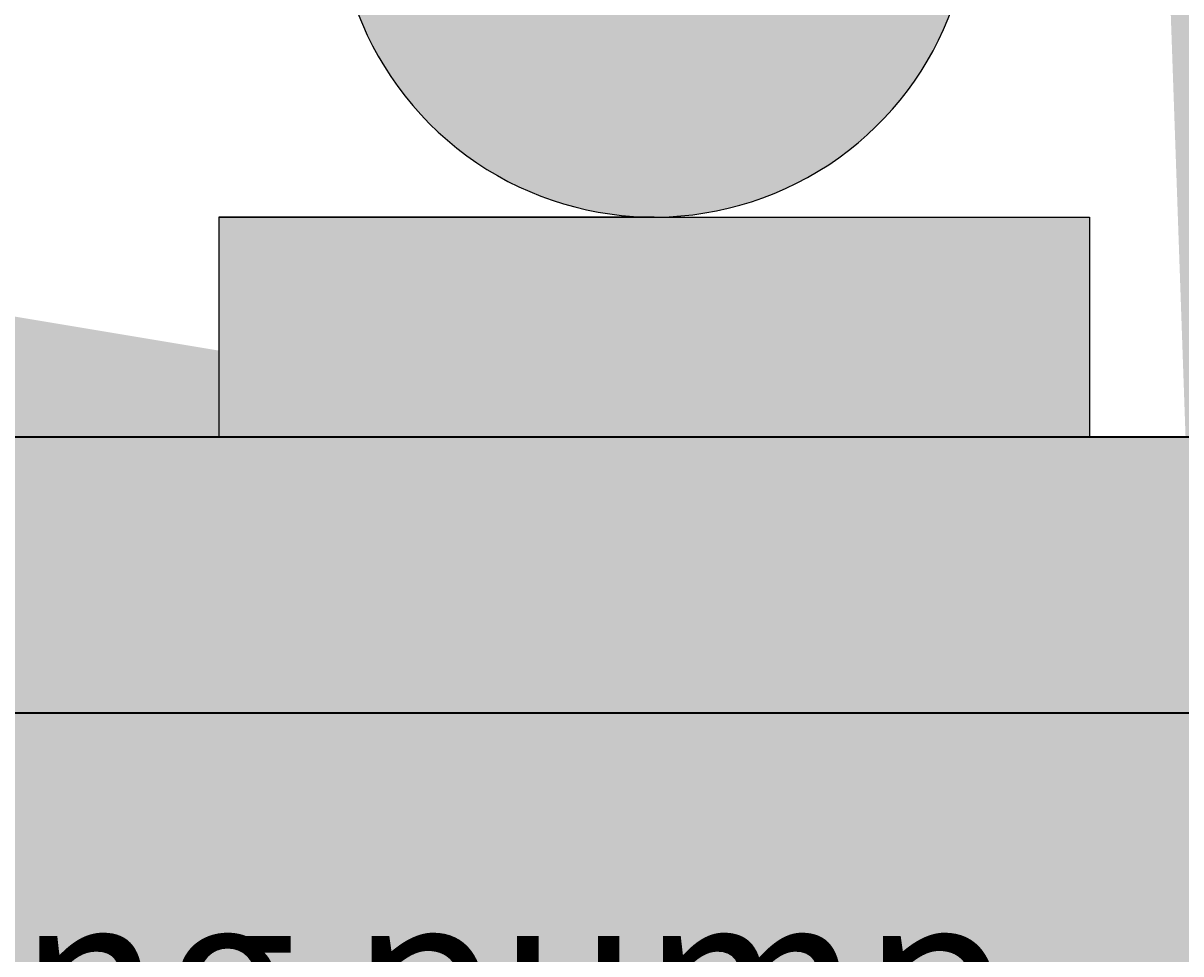
# Model space of a CAD drawing. Units: millimetres. Extents: x -22994 to 29398, y -19990 to 20176.
# Tile 10 of 135: x 32 to 58, y 5 to 26. Entities that reach past the tile are written whole.
import ezdxf
from ezdxf import colors
from ezdxf.entities.mleader import LeaderData, LeaderLine
from ezdxf.math import Vec2, Vec3

# ---------------------------------------------------------------- set-up
doc = ezdxf.new("R2010")
doc.units = ezdxf.units.MM
doc.header["$MEASUREMENT"] = 0
for name, color, linetype, lineweight in [('M-ANNO-TEXT', 7, 'Continuous', 25), ('M-DIMS', 2, 'Continuous', 18), ('M-EQPM', 7, 'Continuous', 25), ('M-EQPM-PATT', 7, 'Continuous', 18), ('S-FNDN', 7, 'Continuous', 35)]:
    doc.layers.add(name, color=color, linetype=linetype, lineweight=lineweight)
doc.styles.get("Standard").update_dxf_attribs({"font": 'arial.ttf'})
doc.dimstyles.get("Standard").update_dxf_attribs({"dimtxt": 0.18, "dimasz": 10000, "dimexe": 0.18, "dimexo": 0.0625, "dimgap": 0.09, "dimtad": 0, "dimtih": 1, "dimtoh": 1, "dimdec": 0, "dimzin": 0, "dimdsep": 46, "dimtxsty": 'Standard', "dimcen": 0.09, "dimadec": 0, "dimazin": 0, "dimtfac": 1, "dimtdec": 0, "dimtofl": 0, "dimtmove": 0, "dimatfit": 3, "dimfxl": 1, "dimtolj": 1, "dimtzin": 0, "dimlwd": 30, "dimarcsym": 0})

# ---------------------------------------------------------------- blocks, each defined once
blk = doc.blocks.new('*D2')
at = {"layer": 'Defpoints', "color": 0, "transparency": 16777216}
for p in [(6.677, 10.271), (290.852, 10.271), (290.852, -5.079)]:
    blk.add_point(p, dxfattribs=at)
at = {"layer": 'M-DIMS', "color": 0, "lineweight": -2, "transparency": 16777216}
for p, q in [((6.677, 10.209), (6.677, -5.259)), ((290.852, 10.209), (290.852, -5.259))]:
    blk.add_line(p, q, dxfattribs=at)
at = {"layer": 'M-DIMS', "color": 0, "lineweight": 30, "transparency": 16777216}
for p, q in [((-9993.323, -5.079), (-19993.323, -5.079)), ((10290.852, -5.079), (20290.852, -5.079))]:
    blk.add_line(p, q, dxfattribs=at)
at = {"layer": 'M-DIMS', "color": 0, "transparency": 16777216}
for points in [[(-9993.323, 1661.588), (-9993.323, -1671.745), (6.677, -5.079)], [(10290.852, 1661.588), (10290.852, -1671.745), (290.852, -5.079)]]:
    blk.add_solid(points, dxfattribs=at)
at = {"layer": 'M-DIMS', "color": 0, "transparency": 16777216, "insert": (148.765, -5.079), "char_height": 0.18, "attachment_point": 5}
blk.add_mtext('\\A1;284.2', dxfattribs=at)
blk = doc.blocks.new('*D3')
at = {"layer": 'Defpoints', "color": 0, "transparency": 16777216}
for p in [(110.265, 204.165), (110.265, 176.366), (95.833, 127.967)]:
    blk.add_point(p, dxfattribs=at)
at = {"layer": 'M-DIMS', "color": 0, "lineweight": -2, "transparency": 16777216}
for p, q in [((95.833, 128.03), (95.833, 204.345)), ((110.265, 176.429), (110.265, 204.345))]:
    blk.add_line(p, q, dxfattribs=at)
at = {"layer": 'M-DIMS', "color": 0, "lineweight": 30, "transparency": 16777216}
for p, q in [((-9904.167, 204.165), (-19904.167, 204.165)), ((10110.265, 204.165), (20110.265, 204.165))]:
    blk.add_line(p, q, dxfattribs=at)
at = {"layer": 'M-DIMS', "color": 0, "transparency": 16777216}
for points in [[(-9904.167, 1870.832), (-9904.167, -1462.501), (95.833, 204.165)], [(10110.265, 1870.832), (10110.265, -1462.501), (110.265, 204.165)]]:
    blk.add_solid(points, dxfattribs=at)
at = {"layer": 'M-DIMS', "color": 0, "transparency": 16777216, "insert": (103.049, 204.165), "char_height": 0.18, "attachment_point": 5}
blk.add_mtext('\\A1;14.432', dxfattribs=at)
blk = doc.blocks.new('*D4')
at = {"layer": 'Defpoints', "color": 0, "transparency": 16777216}
for p in [(116.265, 204.165), (110.265, 176.366), (116.265, 176.366)]:
    blk.add_point(p, dxfattribs=at)
at = {"layer": 'M-DIMS', "color": 0, "lineweight": -2, "transparency": 16777216}
for p, q in [((110.265, 176.429), (110.265, 204.345)), ((116.265, 176.429), (116.265, 204.345))]:
    blk.add_line(p, q, dxfattribs=at)
at = {"layer": 'M-DIMS', "color": 0, "lineweight": 30, "transparency": 16777216}
for p, q in [((-9889.735, 204.165), (-19889.735, 204.165)), ((10116.265, 204.165), (20116.265, 204.165))]:
    blk.add_line(p, q, dxfattribs=at)
at = {"layer": 'M-DIMS', "color": 0, "transparency": 16777216}
for points in [[(-9889.735, 1870.832), (-9889.735, -1462.501), (110.265, 204.165)], [(10116.265, 1870.832), (10116.265, -1462.501), (116.265, 204.165)]]:
    blk.add_solid(points, dxfattribs=at)
at = {"layer": 'M-DIMS', "color": 0, "transparency": 16777216, "insert": (113.265, 204.165), "char_height": 0.18, "attachment_point": 5}
blk.add_mtext('\\A1;6', dxfattribs=at)
blk = doc.blocks.new('*D5')
at = {"layer": 'Defpoints', "color": 0, "transparency": 16777216}
for p in [(181.265, 204.165), (116.265, 176.366), (181.265, 176.366)]:
    blk.add_point(p, dxfattribs=at)
at = {"layer": 'M-DIMS', "color": 0, "lineweight": -2, "transparency": 16777216}
for p, q in [((116.265, 176.429), (116.265, 204.345)), ((181.265, 176.429), (181.265, 204.345))]:
    blk.add_line(p, q, dxfattribs=at)
at = {"layer": 'M-DIMS', "color": 0, "lineweight": 30, "transparency": 16777216}
for p, q in [((-9883.735, 204.165), (-19883.735, 204.165)), ((10181.265, 204.165), (20181.265, 204.165))]:
    blk.add_line(p, q, dxfattribs=at)
at = {"layer": 'M-DIMS', "color": 0, "transparency": 16777216}
for points in [[(-9883.735, 1870.832), (-9883.735, -1462.501), (116.265, 204.165)], [(10181.265, 1870.832), (10181.265, -1462.501), (181.265, 204.165)]]:
    blk.add_solid(points, dxfattribs=at)
at = {"layer": 'M-DIMS', "color": 0, "transparency": 16777216, "insert": (148.765, 204.165), "char_height": 0.18, "attachment_point": 5}
blk.add_mtext('\\A1;65', dxfattribs=at)
blk = doc.blocks.new('*D6')
at = {"layer": 'Defpoints', "color": 0, "transparency": 16777216}
for p in [(187.265, 204.165), (181.265, 176.366), (187.265, 176.366)]:
    blk.add_point(p, dxfattribs=at)
at = {"layer": 'M-DIMS', "color": 0, "lineweight": -2, "transparency": 16777216}
for p, q in [((181.265, 176.429), (181.265, 204.345)), ((187.265, 176.429), (187.265, 204.345))]:
    blk.add_line(p, q, dxfattribs=at)
at = {"layer": 'M-DIMS', "color": 0, "lineweight": 30, "transparency": 16777216}
for p, q in [((-9818.735, 204.165), (-19818.735, 204.165)), ((10187.265, 204.165), (20187.265, 204.165))]:
    blk.add_line(p, q, dxfattribs=at)
at = {"layer": 'M-DIMS', "color": 0, "transparency": 16777216}
for points in [[(-9818.735, 1870.832), (-9818.735, -1462.501), (181.265, 204.165)], [(10187.265, 1870.832), (10187.265, -1462.501), (187.265, 204.165)]]:
    blk.add_solid(points, dxfattribs=at)
at = {"layer": 'M-DIMS', "color": 0, "transparency": 16777216, "insert": (184.265, 204.165), "char_height": 0.18, "attachment_point": 5}
blk.add_mtext('\\A1;6', dxfattribs=at)
blk = doc.blocks.new('*D7')
at = {"layer": 'Defpoints', "color": 0, "transparency": 16777216}
for p in [(201.697, 204.165), (187.265, 176.366), (201.697, 127.967)]:
    blk.add_point(p, dxfattribs=at)
at = {"layer": 'M-DIMS', "color": 0, "lineweight": -2, "transparency": 16777216}
for p, q in [((187.265, 176.429), (187.265, 204.345)), ((201.697, 128.03), (201.697, 204.345))]:
    blk.add_line(p, q, dxfattribs=at)
at = {"layer": 'M-DIMS', "color": 0, "lineweight": 30, "transparency": 16777216}
for p, q in [((-9812.735, 204.165), (-19812.735, 204.165)), ((10201.697, 204.165), (20201.697, 204.165))]:
    blk.add_line(p, q, dxfattribs=at)
at = {"layer": 'M-DIMS', "color": 0, "transparency": 16777216}
for points in [[(-9812.735, 1870.832), (-9812.735, -1462.501), (187.265, 204.165)], [(10201.697, 1870.832), (10201.697, -1462.501), (201.697, 204.165)]]:
    blk.add_solid(points, dxfattribs=at)
at = {"layer": 'M-DIMS', "color": 0, "transparency": 16777216, "insert": (194.481, 204.165), "char_height": 0.18, "attachment_point": 5}
blk.add_mtext('\\A1;14.432', dxfattribs=at)
blk = doc.blocks.new('*D8')
at = {"layer": 'Defpoints', "color": 0, "transparency": 16777216}
for p in [(227.648, 204.165), (227.648, 146.73), (201.697, 127.967)]:
    blk.add_point(p, dxfattribs=at)
at = {"layer": 'M-DIMS', "color": 0, "lineweight": -2, "transparency": 16777216}
for p, q in [((201.697, 128.03), (201.697, 204.345)), ((227.648, 146.792), (227.648, 204.345))]:
    blk.add_line(p, q, dxfattribs=at)
at = {"layer": 'M-DIMS', "color": 0, "lineweight": 30, "transparency": 16777216}
for p, q in [((-9798.303, 204.165), (-19798.303, 204.165)), ((10227.648, 204.165), (20227.648, 204.165))]:
    blk.add_line(p, q, dxfattribs=at)
at = {"layer": 'M-DIMS', "color": 0, "transparency": 16777216}
for points in [[(-9798.303, 1870.832), (-9798.303, -1462.501), (201.697, 204.165)], [(10227.648, 1870.832), (10227.648, -1462.501), (227.648, 204.165)]]:
    blk.add_solid(points, dxfattribs=at)
at = {"layer": 'M-DIMS', "color": 0, "transparency": 16777216, "insert": (214.673, 204.165), "char_height": 0.18, "attachment_point": 5}
blk.add_mtext('\\A1;25.95', dxfattribs=at)
blk = doc.blocks.new('*D9')
at = {"layer": 'Defpoints', "color": 0, "transparency": 16777216}
for p in [(187.265, 176.366), (306.202, 176.366), (290.852, 10.271)]:
    blk.add_point(p, dxfattribs=at)
at = {"layer": 'M-DIMS', "color": 0, "lineweight": 30, "transparency": 16777216}
for p, q in [((306.202, 10176.366), (306.202, 20176.366)), ((306.202, -9989.729), (306.202, -19989.729))]:
    blk.add_line(p, q, dxfattribs=at)
at = {"layer": 'M-DIMS', "color": 0, "lineweight": -2, "transparency": 16777216}
for p, q in [((187.327, 176.366), (306.382, 176.366)), ((290.915, 10.271), (306.382, 10.271))]:
    blk.add_line(p, q, dxfattribs=at)
at = {"layer": 'M-DIMS', "color": 0, "transparency": 16777216}
for points in [[(-1360.465, 10176.366), (1972.869, 10176.366), (306.202, 176.366)], [(-1360.465, -9989.729), (1972.869, -9989.729), (306.202, 10.271)]]:
    blk.add_solid(points, dxfattribs=at)
at = {"layer": 'M-DIMS', "color": 0, "transparency": 16777216, "insert": (306.202, 93.319), "char_height": 0.18, "attachment_point": 5}
blk.add_mtext('\\A1;166.1', dxfattribs=at)
blk = doc.blocks.new('*D10')
at = {"layer": 'Defpoints', "color": 0, "transparency": 16777216}
for p in [(125.65, 136.071), (133.346, 136.071), (133.346, -5.079)]:
    blk.add_point(p, dxfattribs=at)
at = {"layer": 'M-DIMS', "color": 0, "lineweight": -2, "transparency": 16777216}
for p, q in [((125.65, 136.009), (125.65, -5.259)), ((133.346, 136.009), (133.346, -5.259))]:
    blk.add_line(p, q, dxfattribs=at)
at = {"layer": 'M-DIMS', "color": 0, "lineweight": 30, "transparency": 16777216}
for p, q in [((-9874.35, -5.079), (-19874.35, -5.079)), ((10133.346, -5.079), (20133.346, -5.079))]:
    blk.add_line(p, q, dxfattribs=at)
at = {"layer": 'M-DIMS', "color": 0, "transparency": 16777216}
for points in [[(-9874.35, 1661.588), (-9874.35, -1671.745), (125.65, -5.079)], [(10133.346, 1661.588), (10133.346, -1671.745), (133.346, -5.079)]]:
    blk.add_solid(points, dxfattribs=at)
at = {"layer": 'M-DIMS', "color": 0, "transparency": 16777216, "insert": (129.498, -5.079), "char_height": 0.18, "attachment_point": 5}
blk.add_mtext('\\A1;7.696', dxfattribs=at)
blk = doc.blocks.new('*D11')
at = {"layer": 'Defpoints', "color": 0, "transparency": 16777216}
for p in [(133.346, 136.071), (135.65, 136.071), (135.65, -5.079)]:
    blk.add_point(p, dxfattribs=at)
at = {"layer": 'M-DIMS', "color": 0, "lineweight": -2, "transparency": 16777216}
for p, q in [((133.346, 136.009), (133.346, -5.259)), ((135.65, 136.009), (135.65, -5.259))]:
    blk.add_line(p, q, dxfattribs=at)
at = {"layer": 'M-DIMS', "color": 0, "lineweight": 30, "transparency": 16777216}
for p, q in [((-9866.654, -5.079), (-19866.654, -5.079)), ((10135.65, -5.079), (20135.65, -5.079))]:
    blk.add_line(p, q, dxfattribs=at)
at = {"layer": 'M-DIMS', "color": 0, "transparency": 16777216}
for points in [[(-9866.654, 1661.588), (-9866.654, -1671.745), (133.346, -5.079)], [(10135.65, 1661.588), (10135.65, -1671.745), (135.65, -5.079)]]:
    blk.add_solid(points, dxfattribs=at)
at = {"layer": 'M-DIMS', "color": 0, "transparency": 16777216, "insert": (134.498, -5.079), "char_height": 0.18, "attachment_point": 5}
blk.add_mtext('\\A1;2.304', dxfattribs=at)
blk = doc.blocks.new('*D12')
at = {"layer": 'Defpoints', "color": 0, "transparency": 16777216}
for p in [(135.65, 136.071), (145.65, 136.071), (145.65, -5.079)]:
    blk.add_point(p, dxfattribs=at)
at = {"layer": 'M-DIMS', "color": 0, "lineweight": -2, "transparency": 16777216}
for p, q in [((135.65, 136.009), (135.65, -5.259)), ((145.65, 136.009), (145.65, -5.259))]:
    blk.add_line(p, q, dxfattribs=at)
at = {"layer": 'M-DIMS', "color": 0, "lineweight": 30, "transparency": 16777216}
for p, q in [((-9864.35, -5.079), (-19864.35, -5.079)), ((10145.65, -5.079), (20145.65, -5.079))]:
    blk.add_line(p, q, dxfattribs=at)
at = {"layer": 'M-DIMS', "color": 0, "transparency": 16777216}
for points in [[(-9864.35, 1661.588), (-9864.35, -1671.745), (135.65, -5.079)], [(10145.65, 1661.588), (10145.65, -1671.745), (145.65, -5.079)]]:
    blk.add_solid(points, dxfattribs=at)
at = {"layer": 'M-DIMS', "color": 0, "transparency": 16777216, "insert": (140.65, -5.079), "char_height": 0.18, "attachment_point": 5}
blk.add_mtext('\\A1;10', dxfattribs=at)
blk = doc.blocks.new('*D13')
at = {"layer": 'Defpoints', "color": 0, "transparency": 16777216}
for p in [(145.65, 136.071), (155.65, 136.071), (155.65, -5.079)]:
    blk.add_point(p, dxfattribs=at)
at = {"layer": 'M-DIMS', "color": 0, "lineweight": -2, "transparency": 16777216}
for p, q in [((145.65, 136.009), (145.65, -5.259)), ((155.65, 136.009), (155.65, -5.259))]:
    blk.add_line(p, q, dxfattribs=at)
at = {"layer": 'M-DIMS', "color": 0, "lineweight": 30, "transparency": 16777216}
for p, q in [((-9854.35, -5.079), (-19854.35, -5.079)), ((10155.65, -5.079), (20155.65, -5.079))]:
    blk.add_line(p, q, dxfattribs=at)
at = {"layer": 'M-DIMS', "color": 0, "transparency": 16777216}
for points in [[(-9854.35, 1661.588), (-9854.35, -1671.745), (145.65, -5.079)], [(10155.65, 1661.588), (10155.65, -1671.745), (155.65, -5.079)]]:
    blk.add_solid(points, dxfattribs=at)
at = {"layer": 'M-DIMS', "color": 0, "transparency": 16777216, "insert": (150.65, -5.079), "char_height": 0.18, "attachment_point": 5}
blk.add_mtext('\\A1;10', dxfattribs=at)
blk = doc.blocks.new('*D14')
at = {"layer": 'Defpoints', "color": 0, "transparency": 16777216}
for p in [(155.65, 136.071), (165.65, 136.071), (165.65, -5.079)]:
    blk.add_point(p, dxfattribs=at)
at = {"layer": 'M-DIMS', "color": 0, "lineweight": -2, "transparency": 16777216}
for p, q in [((155.65, 136.009), (155.65, -5.259)), ((165.65, 136.009), (165.65, -5.259))]:
    blk.add_line(p, q, dxfattribs=at)
at = {"layer": 'M-DIMS', "color": 0, "lineweight": 30, "transparency": 16777216}
for p, q in [((-9844.35, -5.079), (-19844.35, -5.079)), ((10165.65, -5.079), (20165.65, -5.079))]:
    blk.add_line(p, q, dxfattribs=at)
at = {"layer": 'M-DIMS', "color": 0, "transparency": 16777216}
for points in [[(-9844.35, 1661.588), (-9844.35, -1671.745), (155.65, -5.079)], [(10165.65, 1661.588), (10165.65, -1671.745), (165.65, -5.079)]]:
    blk.add_solid(points, dxfattribs=at)
at = {"layer": 'M-DIMS', "color": 0, "transparency": 16777216, "insert": (160.65, -5.079), "char_height": 0.18, "attachment_point": 5}
blk.add_mtext('\\A1;10', dxfattribs=at)
blk = doc.blocks.new('*D15')
at = {"layer": 'Defpoints', "color": 0, "transparency": 16777216}
for p in [(173.346, 154.788), (173.346, 136.071), (306.202, 136.071)]:
    blk.add_point(p, dxfattribs=at)
at = {"layer": 'M-DIMS', "color": 0, "lineweight": 30, "transparency": 16777216}
for p, q in [((306.202, 10154.788), (306.202, 20154.788)), ((306.202, -9863.929), (306.202, -19863.929))]:
    blk.add_line(p, q, dxfattribs=at)
at = {"layer": 'M-DIMS', "color": 0, "lineweight": -2, "transparency": 16777216}
for p, q in [((173.408, 154.788), (306.382, 154.788)), ((173.408, 136.071), (306.382, 136.071))]:
    blk.add_line(p, q, dxfattribs=at)
at = {"layer": 'M-DIMS', "color": 0, "transparency": 16777216}
for points in [[(-1360.465, 10154.788), (1972.869, 10154.788), (306.202, 154.788)], [(-1360.465, -9863.929), (1972.869, -9863.929), (306.202, 136.071)]]:
    blk.add_solid(points, dxfattribs=at)
at = {"layer": 'M-DIMS', "color": 0, "transparency": 16777216, "insert": (306.202, 145.43), "char_height": 0.18, "attachment_point": 5}
blk.add_mtext('\\A1;18.717', dxfattribs=at)
blk = doc.blocks.new('*D16')
at = {"layer": 'Defpoints', "color": 0, "transparency": 16777216}
for p in [(120.17, 204.165), (110.466, 48.035), (120.17, 48.035)]:
    blk.add_point(p, dxfattribs=at)
at = {"layer": 'M-DIMS', "color": 0, "lineweight": -2, "transparency": 16777216}
for p, q in [((110.466, 48.097), (110.466, 204.345)), ((120.17, 48.097), (120.17, 204.345))]:
    blk.add_line(p, q, dxfattribs=at)
at = {"layer": 'M-DIMS', "color": 0, "lineweight": 30, "transparency": 16777216}
for p, q in [((-9889.534, 204.165), (-19889.534, 204.165)), ((10120.17, 204.165), (20120.17, 204.165))]:
    blk.add_line(p, q, dxfattribs=at)
at = {"layer": 'M-DIMS', "color": 0, "transparency": 16777216}
for points in [[(-9889.534, 1870.832), (-9889.534, -1462.501), (110.466, 204.165)], [(10120.17, 1870.832), (10120.17, -1462.501), (120.17, 204.165)]]:
    blk.add_solid(points, dxfattribs=at)
at = {"layer": 'M-DIMS', "color": 0, "transparency": 16777216, "insert": (115.318, 204.165), "char_height": 0.18, "attachment_point": 5}
blk.add_mtext('\\A1;9.704', dxfattribs=at)
blk = doc.blocks.new('*D17')
at = {"layer": 'Defpoints', "color": 0, "transparency": 16777216}
for p in [(126.17, 204.165), (120.17, 48.035), (126.17, 48.035)]:
    blk.add_point(p, dxfattribs=at)
at = {"layer": 'M-DIMS', "color": 0, "lineweight": -2, "transparency": 16777216}
for p, q in [((120.17, 48.097), (120.17, 204.345)), ((126.17, 48.097), (126.17, 204.345))]:
    blk.add_line(p, q, dxfattribs=at)
at = {"layer": 'M-DIMS', "color": 0, "lineweight": 30, "transparency": 16777216}
for p, q in [((-9879.83, 204.165), (-19879.83, 204.165)), ((10126.17, 204.165), (20126.17, 204.165))]:
    blk.add_line(p, q, dxfattribs=at)
at = {"layer": 'M-DIMS', "color": 0, "transparency": 16777216}
for points in [[(-9879.83, 1870.832), (-9879.83, -1462.501), (120.17, 204.165)], [(10126.17, 1870.832), (10126.17, -1462.501), (126.17, 204.165)]]:
    blk.add_solid(points, dxfattribs=at)
at = {"layer": 'M-DIMS', "color": 0, "transparency": 16777216, "insert": (123.17, 204.165), "char_height": 0.18, "attachment_point": 5}
blk.add_mtext('\\A1;6', dxfattribs=at)
blk = doc.blocks.new('*D18')
at = {"layer": 'Defpoints', "color": 0, "transparency": 16777216}
for p in [(132.17, 204.165), (126.17, 48.035), (132.17, 48.035)]:
    blk.add_point(p, dxfattribs=at)
at = {"layer": 'M-DIMS', "color": 0, "lineweight": -2, "transparency": 16777216}
for p, q in [((126.17, 48.097), (126.17, 204.345)), ((132.17, 48.097), (132.17, 204.345))]:
    blk.add_line(p, q, dxfattribs=at)
at = {"layer": 'M-DIMS', "color": 0, "lineweight": 30, "transparency": 16777216}
for p, q in [((-9873.83, 204.165), (-19873.83, 204.165)), ((10132.17, 204.165), (20132.17, 204.165))]:
    blk.add_line(p, q, dxfattribs=at)
at = {"layer": 'M-DIMS', "color": 0, "transparency": 16777216}
for points in [[(-9873.83, 1870.832), (-9873.83, -1462.501), (126.17, 204.165)], [(10132.17, 1870.832), (10132.17, -1462.501), (132.17, 204.165)]]:
    blk.add_solid(points, dxfattribs=at)
at = {"layer": 'M-DIMS', "color": 0, "transparency": 16777216, "insert": (129.17, 204.165), "char_height": 0.18, "attachment_point": 5}
blk.add_mtext('\\A1;6', dxfattribs=at)
blk = doc.blocks.new('*D19')
at = {"layer": 'Defpoints', "color": 0, "transparency": 16777216}
for p in [(138.17, 204.165), (132.17, 48.035), (138.17, 48.035)]:
    blk.add_point(p, dxfattribs=at)
at = {"layer": 'M-DIMS', "color": 0, "lineweight": -2, "transparency": 16777216}
for p, q in [((132.17, 48.097), (132.17, 204.345)), ((138.17, 48.097), (138.17, 204.345))]:
    blk.add_line(p, q, dxfattribs=at)
at = {"layer": 'M-DIMS', "color": 0, "lineweight": 30, "transparency": 16777216}
for p, q in [((-9867.83, 204.165), (-19867.83, 204.165)), ((10138.17, 204.165), (20138.17, 204.165))]:
    blk.add_line(p, q, dxfattribs=at)
at = {"layer": 'M-DIMS', "color": 0, "transparency": 16777216}
for points in [[(-9867.83, 1870.832), (-9867.83, -1462.501), (132.17, 204.165)], [(10138.17, 1870.832), (10138.17, -1462.501), (138.17, 204.165)]]:
    blk.add_solid(points, dxfattribs=at)
at = {"layer": 'M-DIMS', "color": 0, "transparency": 16777216, "insert": (135.17, 204.165), "char_height": 0.18, "attachment_point": 5}
blk.add_mtext('\\A1;6', dxfattribs=at)
blk = doc.blocks.new('*D20')
at = {"layer": 'Defpoints', "color": 0, "transparency": 16777216}
for p in [(144.17, 204.165), (138.17, 48.035), (144.17, 48.035)]:
    blk.add_point(p, dxfattribs=at)
at = {"layer": 'M-DIMS', "color": 0, "lineweight": -2, "transparency": 16777216}
for p, q in [((138.17, 48.097), (138.17, 204.345)), ((144.17, 48.097), (144.17, 204.345))]:
    blk.add_line(p, q, dxfattribs=at)
at = {"layer": 'M-DIMS', "color": 0, "lineweight": 30, "transparency": 16777216}
for p, q in [((-9861.83, 204.165), (-19861.83, 204.165)), ((10144.17, 204.165), (20144.17, 204.165))]:
    blk.add_line(p, q, dxfattribs=at)
at = {"layer": 'M-DIMS', "color": 0, "transparency": 16777216}
for points in [[(-9861.83, 1870.832), (-9861.83, -1462.501), (138.17, 204.165)], [(10144.17, 1870.832), (10144.17, -1462.501), (144.17, 204.165)]]:
    blk.add_solid(points, dxfattribs=at)
at = {"layer": 'M-DIMS', "color": 0, "transparency": 16777216, "insert": (141.17, 204.165), "char_height": 0.18, "attachment_point": 5}
blk.add_mtext('\\A1;6', dxfattribs=at)
blk = doc.blocks.new('*D21')
at = {"layer": 'Defpoints', "color": 0, "transparency": 16777216}
for p in [(149.116, 204.165), (144.17, 48.035), (149.116, 48.035)]:
    blk.add_point(p, dxfattribs=at)
at = {"layer": 'M-DIMS', "color": 0, "lineweight": -2, "transparency": 16777216}
for p, q in [((144.17, 48.097), (144.17, 204.345)), ((149.116, 48.097), (149.116, 204.345))]:
    blk.add_line(p, q, dxfattribs=at)
at = {"layer": 'M-DIMS', "color": 0, "lineweight": 30, "transparency": 16777216}
for p, q in [((-9855.83, 204.165), (-19855.83, 204.165)), ((10149.116, 204.165), (20149.116, 204.165))]:
    blk.add_line(p, q, dxfattribs=at)
at = {"layer": 'M-DIMS', "color": 0, "transparency": 16777216}
for points in [[(-9855.83, 1870.832), (-9855.83, -1462.501), (144.17, 204.165)], [(10149.116, 1870.832), (10149.116, -1462.501), (149.116, 204.165)]]:
    blk.add_solid(points, dxfattribs=at)
at = {"layer": 'M-DIMS', "color": 0, "transparency": 16777216, "insert": (146.643, 204.165), "char_height": 0.18, "attachment_point": 5}
blk.add_mtext('\\A1;4.945', dxfattribs=at)
blk = doc.blocks.new('*D22')
at = {"layer": 'Defpoints', "color": 0, "transparency": 16777216}
for p in [(149.116, 30.99), (155.116, 30.99), (155.116, -5.079)]:
    blk.add_point(p, dxfattribs=at)
at = {"layer": 'M-DIMS', "color": 0, "lineweight": -2, "transparency": 16777216}
for p, q in [((149.116, 30.927), (149.116, -5.259)), ((155.116, 30.927), (155.116, -5.259))]:
    blk.add_line(p, q, dxfattribs=at)
at = {"layer": 'M-DIMS', "color": 0, "lineweight": 30, "transparency": 16777216}
for p, q in [((-9850.884, -5.079), (-19850.884, -5.079)), ((10155.116, -5.079), (20155.116, -5.079))]:
    blk.add_line(p, q, dxfattribs=at)
at = {"layer": 'M-DIMS', "color": 0, "transparency": 16777216}
for points in [[(-9850.884, 1661.588), (-9850.884, -1671.745), (149.116, -5.079)], [(10155.116, 1661.588), (10155.116, -1671.745), (155.116, -5.079)]]:
    blk.add_solid(points, dxfattribs=at)
at = {"layer": 'M-DIMS', "color": 0, "transparency": 16777216, "insert": (152.116, -5.079), "char_height": 0.18, "attachment_point": 5}
blk.add_mtext('\\A1;6', dxfattribs=at)
blk = doc.blocks.new('*D23')
at = {"layer": 'Defpoints', "color": 0, "transparency": 16777216}
for p in [(155.116, 30.99), (161.116, 30.99), (161.116, -5.079)]:
    blk.add_point(p, dxfattribs=at)
at = {"layer": 'M-DIMS', "color": 0, "lineweight": -2, "transparency": 16777216}
for p, q in [((155.116, 30.927), (155.116, -5.259)), ((161.116, 30.927), (161.116, -5.259))]:
    blk.add_line(p, q, dxfattribs=at)
at = {"layer": 'M-DIMS', "color": 0, "lineweight": 30, "transparency": 16777216}
for p, q in [((-9844.884, -5.079), (-19844.884, -5.079)), ((10161.116, -5.079), (20161.116, -5.079))]:
    blk.add_line(p, q, dxfattribs=at)
at = {"layer": 'M-DIMS', "color": 0, "transparency": 16777216}
for points in [[(-9844.884, 1661.588), (-9844.884, -1671.745), (155.116, -5.079)], [(10161.116, 1661.588), (10161.116, -1671.745), (161.116, -5.079)]]:
    blk.add_solid(points, dxfattribs=at)
at = {"layer": 'M-DIMS', "color": 0, "transparency": 16777216, "insert": (158.116, -5.079), "char_height": 0.18, "attachment_point": 5}
blk.add_mtext('\\A1;6', dxfattribs=at)
blk = doc.blocks.new('*D24')
at = {"layer": 'Defpoints', "color": 0, "transparency": 16777216}
for p in [(161.116, 30.99), (166.439, 30.99), (166.439, -5.079)]:
    blk.add_point(p, dxfattribs=at)
at = {"layer": 'M-DIMS', "color": 0, "lineweight": -2, "transparency": 16777216}
for p, q in [((161.116, 30.927), (161.116, -5.259)), ((166.439, 30.927), (166.439, -5.259))]:
    blk.add_line(p, q, dxfattribs=at)
at = {"layer": 'M-DIMS', "color": 0, "lineweight": 30, "transparency": 16777216}
for p, q in [((-9838.884, -5.079), (-19838.884, -5.079)), ((10166.439, -5.079), (20166.439, -5.079))]:
    blk.add_line(p, q, dxfattribs=at)
at = {"layer": 'M-DIMS', "color": 0, "transparency": 16777216}
for points in [[(-9838.884, 1661.588), (-9838.884, -1671.745), (161.116, -5.079)], [(10166.439, 1661.588), (10166.439, -1671.745), (166.439, -5.079)]]:
    blk.add_solid(points, dxfattribs=at)
at = {"layer": 'M-DIMS', "color": 0, "transparency": 16777216, "insert": (163.777, -5.079), "char_height": 0.18, "attachment_point": 5}
blk.add_mtext('\\A1;5.323', dxfattribs=at)
blk = doc.blocks.new('*D25')
at = {"layer": 'Defpoints', "color": 0, "transparency": 16777216}
for p in [(166.439, 30.99), (172.439, 30.99), (172.439, -5.079)]:
    blk.add_point(p, dxfattribs=at)
at = {"layer": 'M-DIMS', "color": 0, "lineweight": -2, "transparency": 16777216}
for p, q in [((166.439, 30.927), (166.439, -5.259)), ((172.439, 30.927), (172.439, -5.259))]:
    blk.add_line(p, q, dxfattribs=at)
at = {"layer": 'M-DIMS', "color": 0, "lineweight": 30, "transparency": 16777216}
for p, q in [((-9833.561, -5.079), (-19833.561, -5.079)), ((10172.439, -5.079), (20172.439, -5.079))]:
    blk.add_line(p, q, dxfattribs=at)
at = {"layer": 'M-DIMS', "color": 0, "transparency": 16777216}
for points in [[(-9833.561, 1661.588), (-9833.561, -1671.745), (166.439, -5.079)], [(10172.439, 1661.588), (10172.439, -1671.745), (172.439, -5.079)]]:
    blk.add_solid(points, dxfattribs=at)
at = {"layer": 'M-DIMS', "color": 0, "transparency": 16777216, "insert": (169.439, -5.079), "char_height": 0.18, "attachment_point": 5}
blk.add_mtext('\\A1;6', dxfattribs=at)
blk = doc.blocks.new('*D26')
at = {"layer": 'Defpoints', "color": 0, "transparency": 16777216}
for p in [(172.439, 30.99), (178.439, 30.99), (178.439, -5.079)]:
    blk.add_point(p, dxfattribs=at)
at = {"layer": 'M-DIMS', "color": 0, "lineweight": -2, "transparency": 16777216}
for p, q in [((172.439, 30.927), (172.439, -5.259)), ((178.439, 30.927), (178.439, -5.259))]:
    blk.add_line(p, q, dxfattribs=at)
at = {"layer": 'M-DIMS', "color": 0, "lineweight": 30, "transparency": 16777216}
for p, q in [((-9827.561, -5.079), (-19827.561, -5.079)), ((10178.439, -5.079), (20178.439, -5.079))]:
    blk.add_line(p, q, dxfattribs=at)
at = {"layer": 'M-DIMS', "color": 0, "transparency": 16777216}
for points in [[(-9827.561, 1661.588), (-9827.561, -1671.745), (172.439, -5.079)], [(10178.439, 1661.588), (10178.439, -1671.745), (178.439, -5.079)]]:
    blk.add_solid(points, dxfattribs=at)
at = {"layer": 'M-DIMS', "color": 0, "transparency": 16777216, "insert": (175.439, -5.079), "char_height": 0.18, "attachment_point": 5}
blk.add_mtext('\\A1;6', dxfattribs=at)
blk = doc.blocks.new('*D27')
at = {"layer": 'Defpoints', "color": 0, "transparency": 16777216}
for p in [(178.439, 30.99), (188.117, 30.99), (188.117, -5.079)]:
    blk.add_point(p, dxfattribs=at)
at = {"layer": 'M-DIMS', "color": 0, "lineweight": -2, "transparency": 16777216}
for p, q in [((178.439, 30.927), (178.439, -5.259)), ((188.117, 30.927), (188.117, -5.259))]:
    blk.add_line(p, q, dxfattribs=at)
at = {"layer": 'M-DIMS', "color": 0, "lineweight": 30, "transparency": 16777216}
for p, q in [((-9821.561, -5.079), (-19821.561, -5.079)), ((10188.117, -5.079), (20188.117, -5.079))]:
    blk.add_line(p, q, dxfattribs=at)
at = {"layer": 'M-DIMS', "color": 0, "transparency": 16777216}
for points in [[(-9821.561, 1661.588), (-9821.561, -1671.745), (178.439, -5.079)], [(10188.117, 1661.588), (10188.117, -1671.745), (188.117, -5.079)]]:
    blk.add_solid(points, dxfattribs=at)
at = {"layer": 'M-DIMS', "color": 0, "transparency": 16777216, "insert": (183.278, -5.079), "char_height": 0.18, "attachment_point": 5}
blk.add_mtext('\\A1;9.679', dxfattribs=at)
blk = doc.blocks.new('*D28')
at = {"layer": 'Defpoints', "color": 0, "transparency": 16777216}
for p in [(188.117, 48.035), (306.202, 48.035), (188.117, 30.99)]:
    blk.add_point(p, dxfattribs=at)
at = {"layer": 'M-DIMS', "color": 0, "lineweight": 30, "transparency": 16777216}
for p, q in [((306.202, 10048.035), (306.202, 20048.035)), ((306.202, -9969.01), (306.202, -19969.01))]:
    blk.add_line(p, q, dxfattribs=at)
at = {"layer": 'M-DIMS', "color": 0, "lineweight": -2, "transparency": 16777216}
for p, q in [((188.18, 48.035), (306.382, 48.035)), ((188.18, 30.99), (306.382, 30.99))]:
    blk.add_line(p, q, dxfattribs=at)
at = {"layer": 'M-DIMS', "color": 0, "transparency": 16777216}
for points in [[(-1360.465, 10048.035), (1972.869, 10048.035), (306.202, 48.035)], [(-1360.465, -9969.01), (1972.869, -9969.01), (306.202, 30.99)]]:
    blk.add_solid(points, dxfattribs=at)
at = {"layer": 'M-DIMS', "color": 0, "transparency": 16777216, "insert": (306.202, 39.512), "char_height": 0.18, "attachment_point": 5}
blk.add_mtext('\\A1;17.045', dxfattribs=at)
blk = doc.blocks.new('*D29')
at = {"layer": 'Defpoints', "color": 0, "transparency": 16777216}
for p in [(36.801, 80.045), (64.03, 80.045)]:
    blk.add_point(p, dxfattribs=at)
at = {"layer": 'M-DIMS', "color": 0, "lineweight": -2, "transparency": 16777216}
for p, q in [((50.415, 79.955), (50.415, 80.135)), ((50.325, 80.045), (50.505, 80.045))]:
    blk.add_line(p, q, dxfattribs=at)
at = {"layer": 'M-DIMS', "color": 0, "lineweight": 30, "transparency": 16777216}
blk.add_line((20064.03, 80.03), (10064.03, 80.038), dxfattribs=at)
at = {"layer": 'M-DIMS', "color": 0, "transparency": 16777216}
blk.add_solid([(10064.031, 1746.704), (10064.028, -1586.629), (64.03, 80.045)], dxfattribs=at)
at = {"layer": 'M-DIMS', "color": 0, "transparency": 16777216, "insert": (20064.521, 80.03), "char_height": 0.18, "attachment_point": 5}
blk.add_mtext('\\A1;∅27.23', dxfattribs=at)
blk = doc.blocks.new('*D32')
at = {"layer": 'Defpoints', "color": 0, "transparency": 16777216}
for p in [(57.164, 118.614), (52.413, 113.093)]:
    blk.add_point(p, dxfattribs=at)
at = {"layer": 'M-DIMS', "color": 0, "lineweight": -2, "transparency": 16777216}
for p, q in [((57.164, 118.524), (57.164, 118.704)), ((57.074, 118.614), (57.254, 118.614))]:
    blk.add_line(p, q, dxfattribs=at)
at = {"layer": 'M-DIMS', "color": 0, "lineweight": 30, "transparency": 16777216}
for p, q in [((-12992.534, -15047.031), (-6470.06, -7466.969)), ((-22992.534, -15047.031), (-12992.534, -15047.031))]:
    blk.add_line(p, q, dxfattribs=at)
at = {"layer": 'M-DIMS', "color": 0, "transparency": 16777216}
blk.add_solid([(-7733.404, -6379.89), (-5206.717, -8554.048), (52.413, 113.093)], dxfattribs=at)
at = {"layer": 'M-DIMS', "color": 0, "transparency": 16777216, "insert": (-22993.208, -15047.031), "char_height": 0.18, "attachment_point": 5}
blk.add_mtext('\\A1;2X R7.284', dxfattribs=at)
blk = doc.blocks.new('*D37')
at = {"layer": 'Defpoints', "color": 0, "transparency": 16777216}
for p in [(54.834, 118.615), (59.494, 118.614)]:
    blk.add_point(p, dxfattribs=at)
at = {"layer": 'M-DIMS', "color": 0, "lineweight": -2, "transparency": 16777216}
for p, q in [((57.164, 118.524), (57.164, 118.704)), ((57.074, 118.614), (57.254, 118.614))]:
    blk.add_line(p, q, dxfattribs=at)
at = {"layer": 'M-DIMS', "color": 0, "lineweight": 30, "transparency": 16777216}
blk.add_line((20059.493, 116.253), (10059.494, 117.434), dxfattribs=at)
at = {"layer": 'M-DIMS', "color": 0, "transparency": 16777216}
blk.add_solid([(10059.69, 1784.1), (10059.297, -1549.233), (59.494, 118.614)], dxfattribs=at)
at = {"layer": 'M-DIMS', "color": 0, "transparency": 16777216, "insert": (20059.985, 116.253), "char_height": 0.18, "attachment_point": 5}
blk.add_mtext('\\A1;∅4.659', dxfattribs=at)

msp = doc.modelspace()

# ---------------------------------------------------------------- hatches: boundary and pattern name
at = {"layer": 'M-EQPM-PATT'}
h = msp.add_hatch(color=256, dxfattribs=at)
h.set_gradient(color1=(128, 128, 128), color2=(128, 128, 128), tint=1)
h.paths.add_polyline_path([(88.0003, 148.1301), (88.0003, 143.1301), (104.9278, 143.1301), (107.9269, 148.1301)])
h.paths.add_polyline_path([(189.6025, 148.1301), (192.6016, 143.1301), (216.9016, 143.1301, -0.0809736), (216.3148, 146.7296, -0.0309822), (216.4017, 148.1301)])
h.paths.add_polyline_path([(229.9653, 167.6546), (245.0476, 167.6546), (245.0476, 172.6546), (224.9653, 172.6546), (224.9653, 157.741, -0.1116822), (229.9653, 157.8239)])
h.paths.add_polyline_path([(36.3887, 21.6644), (36.3887, 16.6063), (56.3887, 16.6063), (56.3887, 21.6644)])
h = msp.add_hatch(color=256, dxfattribs=at)
h.set_gradient(color1=(242, 103, 34), color2=(242, 103, 34), tint=1, name='CYLINDER')
h.paths.add_polyline_path([(53.5912, 30.0354), (64.8905, 30.0354), (64.8905, 36.2325), (46.3887, 36.2325, 2.6954641)])
h.paths.add_polyline_path([(44.0337, 28.9485, -1), (48.7438, 28.9485, -1)], flags=16)
h.paths.add_polyline_path([(75.6657, 119.7012), (75.6657, 125.8983), (57.1639, 125.8983, 2.6954641), (64.3664, 119.7012)])
h.paths.add_polyline_path([(59.4936, 118.6143, -1), (54.8343, 118.6143, -1)], flags=16)
at = {"layer": 'S-FNDN'}
h = msp.add_hatch(color=256, dxfattribs=at)
h.set_gradient(color1=(241, 235, 31), color2=(244, 238, 81), tint=1, name='CYLINDER')
h.paths.add_polyline_path([(290.852, 16.6063), (201.6967, 16.6063), (95.8327, 16.6063), (81.8485, 16.6063), (82.3691, 10.2713), (290.852, 10.2713)])
h.paths.add_polyline_path([(81.8485, 16.6063), (60.8206, 16.6063), (62.0909, 10.2713), (82.3691, 10.2713)])
h.paths.add_polyline_path([(60.8206, 16.6063), (6.6773, 16.6063), (6.6773, 10.2713), (62.0909, 10.2713)])

# ---------------------------------------------------------------- linework, layer by layer
at = {"layer": 'M-EQPM'}
for p, q in [((46.3887, 21.6644), (36.3887, 21.6644)), ((36.3887, 21.6644), (56.3887, 21.6644)), ((36.3887, 21.6644), (36.3887, 16.6063)), ((56.3887, 21.6644), (56.3887, 16.6063))]:
    msp.add_line(p, q, dxfattribs=at)
msp.add_arc((46.3887, 28.9485), 7.284, 90, 8.58187, dxfattribs=at)
at = {"layer": 'S-FNDN'}
msp.add_lwpolyline([(95.8327, 16.6063), (6.6773, 16.6063), (6.6773, 10.2713), (290.852, 10.2713), (290.852, 16.6063), (201.6967, 16.6063)], dxfattribs=at)

# ---------------------------------------------------------------- dimensions: what is measured, and where the dimension line sits
at = {"layer": 'M-DIMS'}
for base, p1, p2, override, picture, middle in [((306.202, 176.3662), (290.852, 10.2713), (187.2647, 176.3662), {"dimdec": 1, "dimlfac": 1, "dimrnd": 0, "dimzin": 0, "dimdsep": 46, "dimlunit": 2}, '*D9', (306.202, 93.3187)), ((306.202, 136.0713), (173.3459, 154.788), (173.3459, 136.0713), {"dimdec": 3, "dimlfac": 1, "dimrnd": 0, "dimzin": 0, "dimdsep": 46, "dimlunit": 2}, '*D15', (306.202, 145.4297)), ((306.202, 48.0349), (188.1175, 30.9895), (188.1175, 48.0349), {"dimdec": 3, "dimlfac": 1, "dimrnd": 0, "dimzin": 0, "dimdsep": 46, "dimlunit": 2}, '*D28', (306.202, 39.5122))]:
    dim = msp.add_linear_dim(base=base, p1=p1, p2=p2, angle=90, dimstyle='Standard', override=override, dxfattribs=at)
    dim.commit()
    dim.dimension.update_dxf_attribs({"geometry": picture, "text_midpoint": middle})
for base, p1, p2, override, picture, middle in [((110.2647, 204.1654), (95.8327, 127.967), (110.2647, 176.3662), {"dimdec": 3, "dimlfac": 1, "dimrnd": 0, "dimzin": 0, "dimdsep": 46, "dimlunit": 2}, '*D3', (103.0487, 204.1654)), ((116.2647, 204.1654), (110.2647, 176.3662), (116.2647, 176.3662), {"dimdec": 0, "dimlfac": 1, "dimrnd": 0, "dimzin": 0, "dimdsep": 46, "dimlunit": 2}, '*D4', (113.2647, 204.1654)), ((120.1702, 204.1654), (110.4658, 48.0349), (120.1702, 48.0349), {"dimdec": 3, "dimlfac": 1, "dimrnd": 0, "dimzin": 0, "dimdsep": 46, "dimlunit": 2}, '*D16', (115.318, 204.1654)), ((181.2647, 204.1654), (116.2647, 176.3662), (181.2647, 176.3662), {"dimdec": 0, "dimlfac": 1, "dimrnd": 0, "dimzin": 0, "dimdsep": 46, "dimlunit": 2}, '*D5', (148.7647, 204.1654)), ((126.1702, 204.1654), (120.1702, 48.0349), (126.1702, 48.0349), {"dimdec": 0, "dimlfac": 1, "dimrnd": 0, "dimzin": 0, "dimdsep": 46, "dimlunit": 2}, '*D17', (123.1702, 204.1654)), ((132.1702, 204.1654), (126.1702, 48.0349), (132.1702, 48.0349), {"dimdec": 0, "dimlfac": 1, "dimrnd": 0, "dimzin": 0, "dimdsep": 46, "dimlunit": 2}, '*D18', (129.1702, 204.1654)), ((138.1702, 204.1654), (132.1702, 48.0349), (138.1702, 48.0349), {"dimdec": 0, "dimlfac": 1, "dimrnd": 0, "dimzin": 0, "dimdsep": 46, "dimlunit": 2}, '*D19', (135.1702, 204.1654)), ((144.1702, 204.1654), (138.1702, 48.0349), (144.1702, 48.0349), {"dimdec": 0, "dimlfac": 1, "dimrnd": 0, "dimzin": 0, "dimdsep": 46, "dimlunit": 2}, '*D20', (141.1702, 204.1654)), ((149.11567, 204.16539), (144.17023, 48.03494), (149.11567, 48.03494), {"dimdec": 3, "dimlfac": 1, "dimrnd": 0, "dimzin": 0, "dimdsep": 46, "dimlunit": 2}, '*D21', (146.64295, 204.16539)), ((187.2647, 204.1654), (181.2647, 176.3662), (187.2647, 176.3662), {"dimdec": 0, "dimlfac": 1, "dimrnd": 0, "dimzin": 0, "dimdsep": 46, "dimlunit": 2}, '*D6', (184.2647, 204.1654)), ((201.6967, 204.1654), (187.2647, 176.3662), (201.6967, 127.967), {"dimdec": 3, "dimlfac": 1, "dimrnd": 0, "dimzin": 0, "dimdsep": 46, "dimlunit": 2}, '*D7', (194.4807, 204.1654)), ((227.6485, 204.1654), (201.6967, 127.967), (227.6485, 146.7296), {"dimdec": 2, "dimlfac": 1, "dimrnd": 0, "dimzin": 0, "dimdsep": 46, "dimlunit": 2}, '*D8', (214.6726, 204.1654)), ((290.852, -5.0787), (6.6773, 10.2713), (290.852, 10.2713), {"dimdec": 1, "dimlfac": 1, "dimrnd": 0, "dimzin": 0, "dimdsep": 46, "dimlunit": 2}, '*D2', (148.7647, -5.0787)), ((133.3459, -5.0787), (125.6498, 136.0713), (133.3459, 136.0713), {"dimdec": 3, "dimlfac": 1, "dimrnd": 0, "dimzin": 0, "dimdsep": 46, "dimlunit": 2}, '*D10', (129.4978, -5.0787)), ((135.6498, -5.0787), (133.3459, 136.0713), (135.6498, 136.0713), {"dimdec": 3, "dimlfac": 1, "dimrnd": 0, "dimzin": 0, "dimdsep": 46, "dimlunit": 2}, '*D11', (134.4978, -5.0787)), ((145.6498, -5.0787), (135.6498, 136.0713), (145.6498, 136.0713), {"dimdec": 0, "dimlfac": 1, "dimrnd": 0, "dimzin": 0, "dimdsep": 46, "dimlunit": 2}, '*D12', (140.6498, -5.0787)), ((155.6498, -5.0787), (145.6498, 136.0713), (155.6498, 136.0713), {"dimdec": 0, "dimlfac": 1, "dimrnd": 0, "dimzin": 0, "dimdsep": 46, "dimlunit": 2}, '*D13', (150.6498, -5.0787)), ((155.1157, -5.0787), (149.1157, 30.9895), (155.1157, 30.9895), {"dimdec": 0, "dimlfac": 1, "dimrnd": 0, "dimzin": 0, "dimdsep": 46, "dimlunit": 2}, '*D22', (152.1157, -5.0787)), ((161.1157, -5.0787), (155.1157, 30.9895), (161.1157, 30.9895), {"dimdec": 0, "dimlfac": 1, "dimrnd": 0, "dimzin": 0, "dimdsep": 46, "dimlunit": 2}, '*D23', (158.1157, -5.0787)), ((165.6498, -5.0787), (155.6498, 136.0713), (165.6498, 136.0713), {"dimdec": 0, "dimlfac": 1, "dimrnd": 0, "dimzin": 0, "dimdsep": 46, "dimlunit": 2}, '*D14', (160.6498, -5.0787)), ((166.4387, -5.0787), (161.1157, 30.9895), (166.4387, 30.9895), {"dimdec": 3, "dimlfac": 1, "dimrnd": 0, "dimzin": 0, "dimdsep": 46, "dimlunit": 2}, '*D24', (163.7772, -5.0787)), ((172.4387, -5.0787), (166.4387, 30.9895), (172.4387, 30.9895), {"dimdec": 0, "dimlfac": 1, "dimrnd": 0, "dimzin": 0, "dimdsep": 46, "dimlunit": 2}, '*D25', (169.4387, -5.0787)), ((178.4387, -5.0787), (172.4387, 30.9895), (178.4387, 30.9895), {"dimdec": 0, "dimlfac": 1, "dimrnd": 0, "dimzin": 0, "dimdsep": 46, "dimlunit": 2}, '*D26', (175.4387, -5.0787)), ((188.1175, -5.0787), (178.4387, 30.9895), (188.1175, 30.9895), {"dimdec": 3, "dimlfac": 1, "dimrnd": 0, "dimzin": 0, "dimdsep": 46, "dimlunit": 2}, '*D27', (183.2781, -5.0787))]:
    dim = msp.add_linear_dim(base=base, p1=p1, p2=p2, dimstyle='Standard', override=override, dxfattribs=at)
    dim.commit()
    dim.dimension.update_dxf_attribs({"geometry": picture, "text_midpoint": middle})
for p1, p2, override, picture, middle in [((54.8343, 118.6145), (59.4936, 118.614), {"dimdec": 3, "dimlfac": 1, "dimrnd": 0, "dimzin": 0, "dimdsep": 46, "dimlunit": 2}, '*D37', (20059.4934, 116.2531)), ((36.8006, 80.045), (64.0296, 80.045), {"dimdec": 2, "dimlfac": 1, "dimrnd": 0, "dimzin": 0, "dimdsep": 46, "dimlunit": 2}, '*D29', (20064.0296, 80.0303))]:
    dim = msp.add_diameter_dim_2p(p1=p1, p2=p2, dimstyle='Standard', override=override, dxfattribs=at)
    dim.commit()
    dim.dimension.update_dxf_attribs({"geometry": picture, "text_midpoint": middle})
dim = msp.add_radius_dim(center=(57.1639, 118.6143), mpoint=(52.4129, 113.0929), text='2X <>', dimstyle='Standard', override={"dimdec": 3, "dimlfac": 1, "dimrnd": 0, "dimzin": 0, "dimdsep": 46, "dimlunit": 2}, dxfattribs=at)
dim.commit()
dim.dimension.update_dxf_attribs({"geometry": '*D32', "text_midpoint": (-22993.208, -15047.0314)})

# ---------------------------------------------------------------- leaders
at = {"layer": 'M-ANNO-TEXT'}
ml = msp.add_multileader_mtext('Standard', dxfattribs=at)
ml.set_content('Circulating pump', color=256)
ml.set_leader_properties()
ml.build(insert=Vec2(0, 0))
ml.multileader.update_dxf_attribs({"dogleg_length": 0.36, "arrow_head_size": 200})
ctx = ml.context
ctx.base_point, ctx.arrow_head_size, ctx.landing_gap_size, ctx.plane_origin = Vec3(13.008, 3.5951), 200, 0.09, Vec3(56.3887, 19.3615)
ctx.text_align_type = 2
notes = []
notes.append((ctx, [(1, (1, 1, 0), (63.4296, 3.5951), (-1, 0), 8.8146, [(0, [(58.1278, 30.0354)], 0, [])])]))
ctx.mtext.insert, ctx.mtext.alignment, ctx.mtext.flow_direction = Vec3(54.525, 6.1831), 3, 5
for ctx, leaders in notes:
    for number, flags, end, landing, length, lines in leaders:
        leader = LeaderData()
        leader.index, (leader.has_last_leader_line, leader.has_dogleg_vector, leader.attachment_direction) = number, flags
        leader.last_leader_point, leader.dogleg_vector, leader.dogleg_length = Vec3(end), Vec3(landing), length
        for number, points, colour, breaks in lines:
            line = LeaderLine()
            line.index, line.vertices, line.color, line.breaks = number, Vec3.list(points), colors.encode_raw_color(colour), breaks
            leader.lines.append(line)
        ctx.leaders.append(leader)

doc.saveas('drawing.dxf')
